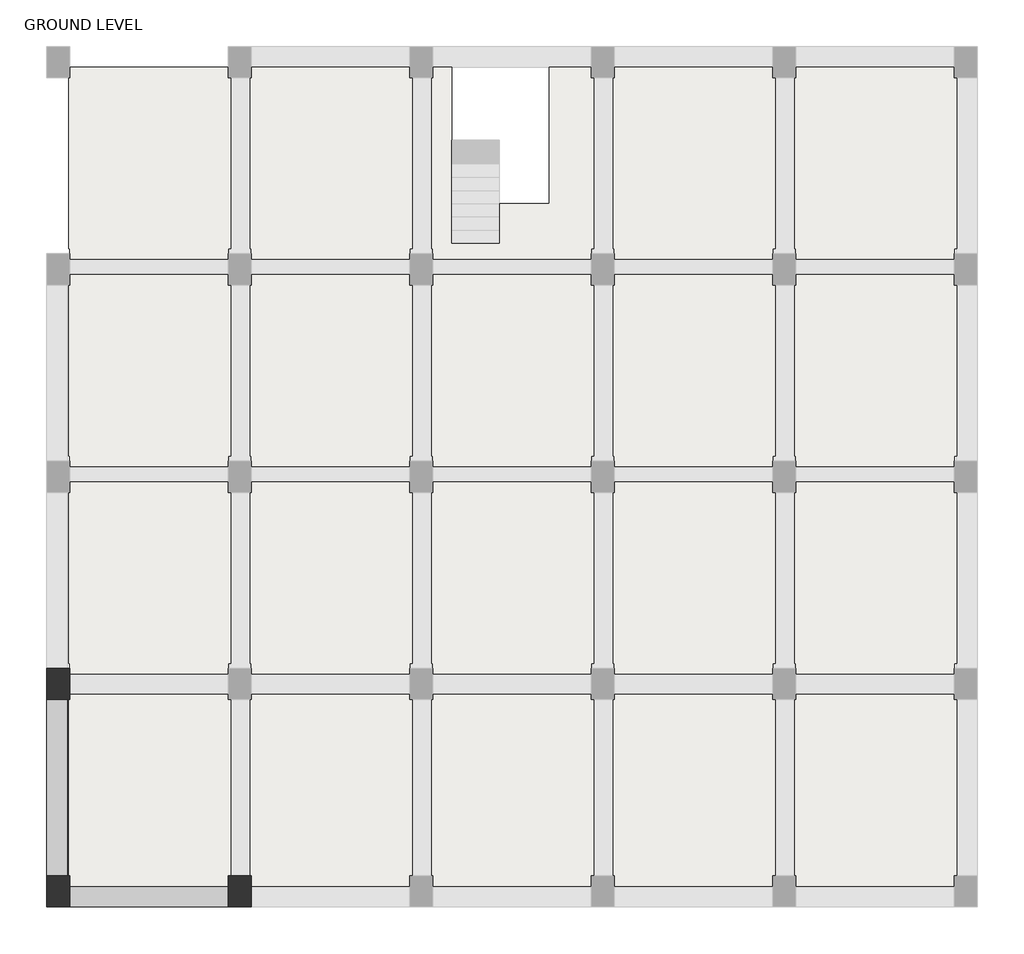
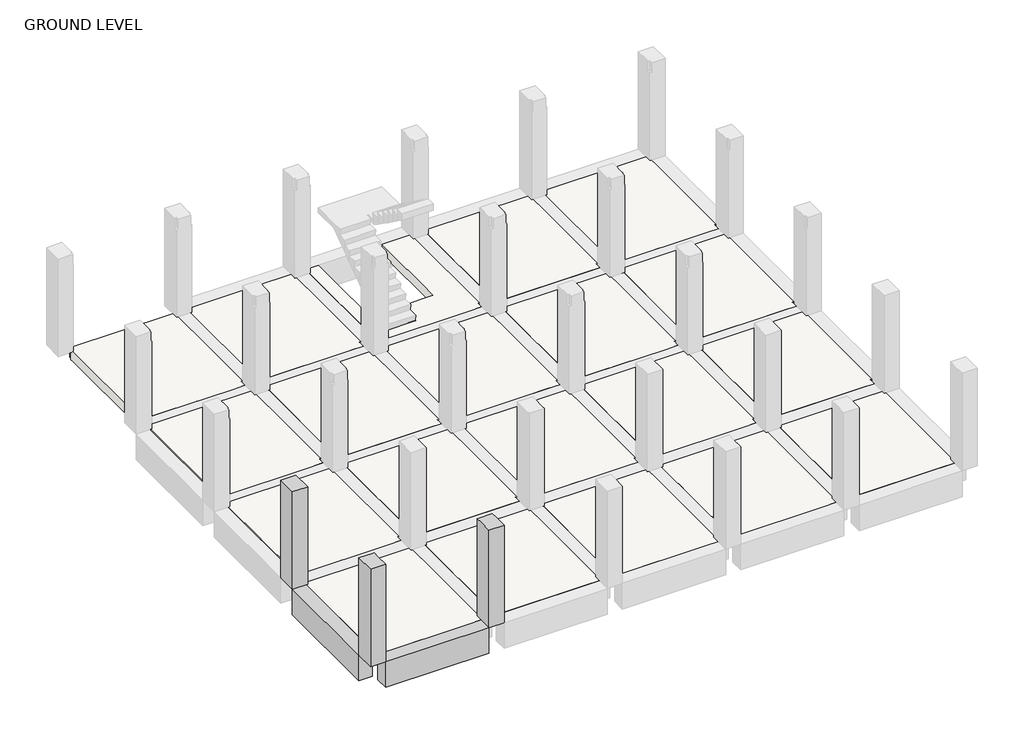
# One storey, part 1 of 3: 20 slabs, 3 columns, 2 beams.
"""IFC4 building model written with IfcOpenShell, lengths in millimetres."""

from ifc_helpers import new_model, si_unit, frame, origin, place, context, project, spatial, polyline, outline, extrude, faceted_brep, element, save

model = new_model("IFC4")

# Units and contexts
model_context = context("Model", 3, world=origin())
ifc_project = project(units=[si_unit("LENGTHUNIT", "METRE", prefix="MILLI")], contexts=[model_context])

# Site, building, storey
site = spatial("IfcSite", under=ifc_project)
building = spatial("IfcBuilding", under=site)
storey = spatial("IfcBuildingStorey", under=building, Name="GROUND LEVEL", Elevation=0.0)

# Beams
placement = place(None, origin())
element("IfcBeam", 1, ObjectType="M_Concrete-Rectangular Beam : 400 x 800mm", at=placement, inside=storey, context=model_context, shape_type="Brep", body=[
    faceted_brep([(-9144.8884094, 3503.1212443, 0.0), (-9144.8884094, 3103.1212443, 0.0), (-6094.8884094, 3103.1212443, 0.0), (-6094.8884094, 3503.1212443, 0.0), (-9144.8884094, 3503.1212443, -800.0), (-9144.8884094, 3503.1212443, -300.0), (-6094.8884094, 3503.1212443, -300.0), (-6094.8884094, 3503.1212443, -800.0), (-9144.8884094, 3103.1212443, -800.0), (-6094.8884094, 3103.1212443, -800.0)], [[[0, 1, 2, 3]], [[4, 5, 0, 3, 6, 7]], [[8, 4, 7, 9]], [[1, 8, 9, 2]], [[1, 0, 5, 4, 8]], [[3, 2, 9, 7, 6]]]),
])
element("IfcBeam", 2, ObjectType="M_Concrete-Rectangular Beam : 400 x 800mm", at=placement, inside=storey, context=model_context, shape_type="SweptSolid", body=[
    extrude(outline(polyline([(-9594.8884094, 7103.1212443), (-9194.8884094, 7103.1212443), (-9194.8884094, 3703.1212443), (-9594.8884094, 3703.1212443), (-9594.8884094, 7103.1212443)])), frame((0.0, 0.0, -800.0), z_axis=(0.0, 0.0, 1.0), x_axis=(1.0, 0.0, 0.0)), (0.0, 0.0, 1.0), 800.0),
])

# Columns
element("IfcColumn", 3, ObjectType="M_Concrete-Rectangular-Column : 450 x 600mm", at=placement, inside=storey, context=model_context, shape_type="Brep", body=[
    faceted_brep([(-9144.8884094, 7703.1212443, 0.0), (-9144.8884094, 7103.1212443, 0.0), (-9594.8884094, 7103.1212443, 0.0), (-9594.8884094, 7703.1212443, 0.0), (-9144.8884094, 7703.1212443, 2748.0), (-9144.8884094, 7703.1212443, 3048.0), (-9144.8884094, 7603.1212443, 3048.0), (-9144.8884094, 7203.1212443, 3048.0), (-9144.8884094, 7103.1212443, 3048.0), (-9144.8884094, 7103.1212443, 2748.0), (-9169.8884094, 7103.1212443, 3048.0), (-9594.8884094, 7103.1212443, 3048.0), (-9594.8884094, 7703.1212443, 3048.0)], [[[0, 1, 2, 3]], [[1, 0, 4, 5, 6, 7, 8, 9]], [[2, 1, 9, 8, 10, 11]], [[3, 2, 11, 12]], [[0, 3, 12, 5, 4]], [[12, 11, 10, 8, 7, 6, 5]]]),
])
element("IfcColumn", 4, ObjectType="M_Concrete-Rectangular-Column : 450 x 600mm", at=placement, inside=storey, context=model_context, shape_type="Brep", body=[
    faceted_brep([(-9144.8884094, 3703.1212443, 0.0), (-9144.8884094, 3103.1212443, 0.0), (-9594.8884094, 3103.1212443, 0.0), (-9594.8884094, 3703.1212443, 0.0), (-9144.8884094, 3703.1212443, 2748.0), (-9144.8884094, 3703.1212443, 3048.0), (-9144.8884094, 3503.1212443, 3048.0), (-9144.8884094, 3103.1212443, 3048.0), (-9594.8884094, 3103.1212443, 3048.0), (-9594.8884094, 3703.1212443, 3048.0), (-9169.8884094, 3703.1212443, 3048.0)], [[[0, 1, 2, 3]], [[1, 0, 4, 5, 6, 7]], [[2, 1, 7, 8]], [[3, 2, 8, 9]], [[0, 3, 9, 10, 5, 4]], [[8, 7, 6, 5, 10, 9]]]),
])
element("IfcColumn", 5, ObjectType="M_Concrete-Rectangular-Column : 450 x 600mm", at=placement, inside=storey, context=model_context, shape_type="Brep", body=[
    faceted_brep([(-5644.8884094, 3703.1212443, 0.0), (-5644.8884094, 3103.1212443, 0.0), (-6094.8884094, 3103.1212443, 0.0), (-6094.8884094, 3703.1212443, 0.0), (-5644.8884094, 3703.1212443, 2748.0), (-5644.8884094, 3703.1212443, 3048.0), (-5644.8884094, 3503.1212443, 3048.0), (-5644.8884094, 3103.1212443, 3048.0), (-6094.8884094, 3103.1212443, 3048.0), (-6094.8884094, 3503.1212443, 3048.0), (-6094.8884094, 3703.1212443, 3048.0), (-6094.8884094, 3703.1212443, 2748.0), (-6044.8884094, 3703.1212443, 3048.0), (-5669.8884094, 3703.1212443, 3048.0)], [[[0, 1, 2, 3]], [[1, 0, 4, 5, 6, 7]], [[2, 1, 7, 8]], [[3, 2, 8, 9, 10, 11]], [[0, 3, 11, 10, 12, 13, 5, 4]], [[8, 7, 6, 5, 13, 12, 10, 9]]]),
])

# Slabs
element("IfcSlab", 6, ObjectType="Generic 300mm", at=placement, inside=storey, context=model_context, shape_type="SweptSolid", body=[
    extrude(outline(polyline([(7955.1115906, 7103.1212443), (7955.1115906, 3703.1212443), (7905.1115906, 3703.1212443), (7905.1115906, 3503.1212443), (7530.1115906, 3503.1212443), (4855.1115906, 3503.1212443), (4855.1115906, 3703.1212443), (4830.1115906, 3703.1212443), (4830.1115906, 7103.1212443), (4855.1115906, 7103.1212443), (4855.1115906, 7203.1212443), (7905.1115906, 7203.1212443), (7905.1115906, 7103.1212443), (7955.1115906, 7103.1212443)])), frame((0.0, 0.0, -300.0), z_axis=(0.0, 0.0, 1.0), x_axis=(1.0, 0.0, 0.0)), (0.0, 0.0, 1.0), 300.0),
])
element("IfcSlab", 7, ObjectType="Generic 300mm", at=placement, inside=storey, context=model_context, shape_type="Brep", body=[
    faceted_brep([(7955.1115906, 11203.1212443, -300.0), (7955.1115906, 11103.1212443, -300.0), (7955.1115906, 7803.1212443, -300.0), (7905.1115906, 7803.1212443, -300.0), (7905.1115906, 7603.1212443, -300.0), (7530.1115906, 7603.1212443, -300.0), (4855.1115906, 7603.1212443, -300.0), (4855.1115906, 7803.1212443, -300.0), (4830.1115906, 7803.1212443, -300.0), (4830.1115906, 11103.1212443, -300.0), (4830.1115906, 11203.1212443, -300.0), (4855.1115906, 11203.1212443, -300.0), (4855.1115906, 11303.1212443, -300.0), (7905.1115906, 11303.1212443, -300.0), (7905.1115906, 11203.1212443, -300.0), (7955.1115906, 11203.1212443, 0.0), (7905.1115906, 11203.1212443, 0.0), (7905.1115906, 11303.1212443, 0.0), (4855.1115906, 11303.1212443, 0.0), (4855.1115906, 11203.1212443, 0.0), (4830.1115906, 11203.1212443, 0.0), (4830.1115906, 11103.1212443, 0.0), (4830.1115906, 7803.1212443, 0.0), (4855.1115906, 7803.1212443, 0.0), (4855.1115906, 7703.1212443, 0.0), (4855.1115906, 7603.1212443, 0.0), (7530.1115906, 7603.1212443, 0.0), (7905.1115906, 7603.1212443, 0.0), (7905.1115906, 7703.1212443, 0.0), (7905.1115906, 7803.1212443, 0.0), (7955.1115906, 7803.1212443, 0.0), (7955.1115906, 11103.1212443, 0.0)], [[[0, 1, 2, 3, 4, 5, 6, 7, 8, 9, 10, 11, 12, 13, 14]], [[15, 16, 17, 18, 19, 20, 21, 22, 23, 24, 25, 26, 27, 28, 29, 30, 31]], [[2, 1, 0, 15, 31, 30]], [[3, 2, 30, 29]], [[4, 3, 29, 28, 27]], [[5, 4, 27, 26]], [[6, 5, 26, 25]], [[7, 6, 25, 24, 23]], [[8, 7, 23, 22]], [[10, 9, 8, 22, 21, 20]], [[11, 10, 20, 19]], [[12, 11, 19, 18]], [[13, 12, 18, 17]], [[14, 13, 17, 16]], [[0, 14, 16, 15]]]),
])
element("IfcSlab", 8, ObjectType="Generic 300mm", at=placement, inside=storey, context=model_context, shape_type="Brep", body=[
    faceted_brep([(4455.1115906, 11203.1212443, -300.0), (4455.1115906, 11103.1212443, -300.0), (4455.1115906, 7803.1212443, -300.0), (4430.1115906, 7803.1212443, -300.0), (4405.1115906, 7803.1212443, -300.0), (4405.1115906, 7603.1212443, -300.0), (4030.1115906, 7603.1212443, -300.0), (1355.1115906, 7603.1212443, -300.0), (1355.1115906, 7803.1212443, -300.0), (1330.1115906, 7803.1212443, -300.0), (1330.1115906, 11103.1212443, -300.0), (1330.1115906, 11203.1212443, -300.0), (1355.1115906, 11203.1212443, -300.0), (1355.1115906, 11303.1212443, -300.0), (4405.1115906, 11303.1212443, -300.0), (4405.1115906, 11203.1212443, -300.0), (4455.1115906, 11203.1212443, 0.0), (4405.1115906, 11203.1212443, 0.0), (4405.1115906, 11303.1212443, 0.0), (1355.1115906, 11303.1212443, 0.0), (1355.1115906, 11203.1212443, 0.0), (1330.1115906, 11203.1212443, 0.0), (1330.1115906, 11103.1212443, 0.0), (1330.1115906, 7803.1212443, 0.0), (1355.1115906, 7803.1212443, 0.0), (1355.1115906, 7703.1212443, 0.0), (1355.1115906, 7603.1212443, 0.0), (4030.1115906, 7603.1212443, 0.0), (4405.1115906, 7603.1212443, 0.0), (4405.1115906, 7703.1212443, 0.0), (4405.1115906, 7803.1212443, 0.0), (4430.1115906, 7803.1212443, 0.0), (4455.1115906, 7803.1212443, 0.0), (4455.1115906, 11103.1212443, 0.0)], [[[0, 1, 2, 3, 4, 5, 6, 7, 8, 9, 10, 11, 12, 13, 14, 15]], [[16, 17, 18, 19, 20, 21, 22, 23, 24, 25, 26, 27, 28, 29, 30, 31, 32, 33]], [[2, 1, 0, 16, 33, 32]], [[4, 3, 2, 32, 31, 30]], [[5, 4, 30, 29, 28]], [[6, 5, 28, 27]], [[7, 6, 27, 26]], [[8, 7, 26, 25, 24]], [[9, 8, 24, 23]], [[11, 10, 9, 23, 22, 21]], [[12, 11, 21, 20]], [[13, 12, 20, 19]], [[14, 13, 19, 18]], [[15, 14, 18, 17]], [[0, 15, 17, 16]]]),
])
element("IfcSlab", 9, ObjectType="Generic 300mm", at=placement, inside=storey, context=model_context, shape_type="Brep", body=[
    faceted_brep([(955.1115906, 11203.1212443, -300.0), (955.1115906, 11103.1212443, -300.0), (955.1115906, 7803.1212443, -300.0), (930.1115906, 7803.1212443, -300.0), (905.1115906, 7803.1212443, -300.0), (905.1115906, 7603.1212443, -300.0), (530.1115906, 7603.1212443, -300.0), (-2144.8884094, 7603.1212443, -300.0), (-2144.8884094, 7803.1212443, -300.0), (-2169.8884094, 7803.1212443, -300.0), (-2169.8884094, 11103.1212443, -300.0), (-2169.8884094, 11203.1212443, -300.0), (-2144.8884094, 11203.1212443, -300.0), (-2144.8884094, 11303.1212443, -300.0), (905.1115906, 11303.1212443, -300.0), (905.1115906, 11203.1212443, -300.0), (955.1115906, 11203.1212443, 0.0), (905.1115906, 11203.1212443, 0.0), (905.1115906, 11303.1212443, 0.0), (-2144.8884094, 11303.1212443, 0.0), (-2144.8884094, 11203.1212443, 0.0), (-2169.8884094, 11203.1212443, 0.0), (-2169.8884094, 11103.1212443, 0.0), (-2169.8884094, 7803.1212443, 0.0), (-2144.8884094, 7803.1212443, 0.0), (-2144.8884094, 7703.1212443, 0.0), (-2144.8884094, 7603.1212443, 0.0), (530.1115906, 7603.1212443, 0.0), (905.1115906, 7603.1212443, 0.0), (905.1115906, 7703.1212443, 0.0), (905.1115906, 7803.1212443, 0.0), (930.1115906, 7803.1212443, 0.0), (955.1115906, 7803.1212443, 0.0), (955.1115906, 11103.1212443, 0.0)], [[[0, 1, 2, 3, 4, 5, 6, 7, 8, 9, 10, 11, 12, 13, 14, 15]], [[16, 17, 18, 19, 20, 21, 22, 23, 24, 25, 26, 27, 28, 29, 30, 31, 32, 33]], [[2, 1, 0, 16, 33, 32]], [[4, 3, 2, 32, 31, 30]], [[5, 4, 30, 29, 28]], [[6, 5, 28, 27]], [[7, 6, 27, 26]], [[8, 7, 26, 25, 24]], [[9, 8, 24, 23]], [[11, 10, 9, 23, 22, 21]], [[12, 11, 21, 20]], [[13, 12, 20, 19]], [[14, 13, 19, 18]], [[15, 14, 18, 17]], [[0, 15, 17, 16]]]),
])
element("IfcSlab", 10, ObjectType="Generic 300mm", at=placement, inside=storey, context=model_context, shape_type="Brep", body=[
    faceted_brep([(-2544.8884094, 11203.1212443, -300.0), (-2544.8884094, 11103.1212443, -300.0), (-2544.8884094, 7803.1212443, -300.0), (-2569.8884094, 7803.1212443, -300.0), (-2594.8884094, 7803.1212443, -300.0), (-2594.8884094, 7603.1212443, -300.0), (-2969.8884094, 7603.1212443, -300.0), (-5644.8884094, 7603.1212443, -300.0), (-5644.8884094, 7803.1212443, -300.0), (-5669.8884094, 7803.1212443, -300.0), (-5669.8884094, 11103.1212443, -300.0), (-5669.8884094, 11203.1212443, -300.0), (-5644.8884094, 11203.1212443, -300.0), (-5644.8884094, 11303.1212443, -300.0), (-2594.8884094, 11303.1212443, -300.0), (-2594.8884094, 11203.1212443, -300.0), (-2544.8884094, 11203.1212443, 0.0), (-2594.8884094, 11203.1212443, 0.0), (-2594.8884094, 11303.1212443, 0.0), (-5644.8884094, 11303.1212443, 0.0), (-5644.8884094, 11203.1212443, 0.0), (-5669.8884094, 11203.1212443, 0.0), (-5669.8884094, 11103.1212443, 0.0), (-5669.8884094, 7803.1212443, 0.0), (-5644.8884094, 7803.1212443, 0.0), (-5644.8884094, 7703.1212443, 0.0), (-5644.8884094, 7603.1212443, 0.0), (-2969.8884094, 7603.1212443, 0.0), (-2594.8884094, 7603.1212443, 0.0), (-2594.8884094, 7703.1212443, 0.0), (-2594.8884094, 7803.1212443, 0.0), (-2569.8884094, 7803.1212443, 0.0), (-2544.8884094, 7803.1212443, 0.0), (-2544.8884094, 11103.1212443, 0.0)], [[[0, 1, 2, 3, 4, 5, 6, 7, 8, 9, 10, 11, 12, 13, 14, 15]], [[16, 17, 18, 19, 20, 21, 22, 23, 24, 25, 26, 27, 28, 29, 30, 31, 32, 33]], [[2, 1, 0, 16, 33, 32]], [[4, 3, 2, 32, 31, 30]], [[5, 4, 30, 29, 28]], [[6, 5, 28, 27]], [[7, 6, 27, 26]], [[8, 7, 26, 25, 24]], [[9, 8, 24, 23]], [[11, 10, 9, 23, 22, 21]], [[12, 11, 21, 20]], [[13, 12, 20, 19]], [[14, 13, 19, 18]], [[15, 14, 18, 17]], [[0, 15, 17, 16]]]),
])
element("IfcSlab", 11, ObjectType="Generic 300mm", at=placement, inside=storey, context=model_context, shape_type="Brep", body=[
    faceted_brep([(-6044.8884094, 11203.1212443, -300.0), (-6044.8884094, 11103.1212443, -300.0), (-6044.8884094, 7803.1212443, -300.0), (-6069.8884094, 7803.1212443, -300.0), (-6094.8884094, 7803.1212443, -300.0), (-6094.8884094, 7603.1212443, -300.0), (-6469.8884094, 7603.1212443, -300.0), (-9144.8884094, 7603.1212443, -300.0), (-9144.8884094, 7803.1212443, -300.0), (-9169.8884094, 7803.1212443, -300.0), (-9169.8884094, 11103.1212443, -300.0), (-9169.8884094, 11203.1212443, -300.0), (-9144.8884094, 11203.1212443, -300.0), (-9144.8884094, 11303.1212443, -300.0), (-6094.8884094, 11303.1212443, -300.0), (-6094.8884094, 11203.1212443, -300.0), (-6044.8884094, 11203.1212443, 0.0), (-6094.8884094, 11203.1212443, 0.0), (-6094.8884094, 11303.1212443, 0.0), (-9144.8884094, 11303.1212443, 0.0), (-9144.8884094, 11203.1212443, 0.0), (-9169.8884094, 11203.1212443, 0.0), (-9169.8884094, 11103.1212443, 0.0), (-9169.8884094, 7803.1212443, 0.0), (-9144.8884094, 7803.1212443, 0.0), (-9144.8884094, 7703.1212443, 0.0), (-9144.8884094, 7603.1212443, 0.0), (-6469.8884094, 7603.1212443, 0.0), (-6094.8884094, 7603.1212443, 0.0), (-6094.8884094, 7703.1212443, 0.0), (-6094.8884094, 7803.1212443, 0.0), (-6069.8884094, 7803.1212443, 0.0), (-6044.8884094, 7803.1212443, 0.0), (-6044.8884094, 11103.1212443, 0.0)], [[[0, 1, 2, 3, 4, 5, 6, 7, 8, 9, 10, 11, 12, 13, 14, 15]], [[16, 17, 18, 19, 20, 21, 22, 23, 24, 25, 26, 27, 28, 29, 30, 31, 32, 33]], [[2, 1, 0, 16, 33, 32]], [[4, 3, 2, 32, 31, 30]], [[5, 4, 30, 29, 28]], [[6, 5, 28, 27]], [[7, 6, 27, 26]], [[8, 7, 26, 25, 24]], [[9, 8, 24, 23]], [[11, 10, 9, 23, 22, 21]], [[12, 11, 21, 20]], [[13, 12, 20, 19]], [[14, 13, 19, 18]], [[15, 14, 18, 17]], [[0, 15, 17, 16]]]),
])
element("IfcSlab", 12, ObjectType="Generic 300mm", at=placement, inside=storey, context=model_context, shape_type="Brep", body=[
    faceted_brep([(-6044.8884094, 7103.1212443, -300.0), (-6044.8884094, 3703.1212443, -300.0), (-6069.8884094, 3703.1212443, -300.0), (-6094.8884094, 3703.1212443, -300.0), (-6094.8884094, 3503.1212443, -300.0), (-6469.8884094, 3503.1212443, -300.0), (-9144.8884094, 3503.1212443, -300.0), (-9144.8884094, 3703.1212443, -300.0), (-9169.8884094, 3703.1212443, -300.0), (-9169.8884094, 7103.1212443, -300.0), (-9144.8884094, 7103.1212443, -300.0), (-9144.8884094, 7203.1212443, -300.0), (-6094.8884094, 7203.1212443, -300.0), (-6094.8884094, 7103.1212443, -300.0), (-6069.8884094, 7103.1212443, -300.0), (-6044.8884094, 7103.1212443, 0.0), (-6094.8884094, 7103.1212443, 0.0), (-6094.8884094, 7203.1212443, 0.0), (-9144.8884094, 7203.1212443, 0.0), (-9144.8884094, 7103.1212443, 0.0), (-9169.8884094, 7103.1212443, 0.0), (-9169.8884094, 3703.1212443, 0.0), (-9144.8884094, 3703.1212443, 0.0), (-9144.8884094, 3503.1212443, 0.0), (-6469.8884094, 3503.1212443, 0.0), (-6094.8884094, 3503.1212443, 0.0), (-6094.8884094, 3703.1212443, 0.0), (-6044.8884094, 3703.1212443, 0.0)], [[[0, 1, 2, 3, 4, 5, 6, 7, 8, 9, 10, 11, 12, 13, 14]], [[15, 16, 17, 18, 19, 20, 21, 22, 23, 24, 25, 26, 27]], [[1, 0, 15, 27]], [[3, 2, 1, 27, 26]], [[4, 3, 26, 25]], [[5, 4, 25, 24]], [[6, 5, 24, 23]], [[7, 6, 23, 22]], [[8, 7, 22, 21]], [[9, 8, 21, 20]], [[10, 9, 20, 19]], [[11, 10, 19, 18]], [[12, 11, 18, 17]], [[13, 12, 17, 16]], [[0, 14, 13, 16, 15]]]),
])
element("IfcSlab", 13, ObjectType="Generic 300mm", at=placement, inside=storey, context=model_context, shape_type="Brep", body=[
    faceted_brep([(-2544.8884094, 7103.1212443, -300.0), (-2544.8884094, 3703.1212443, -300.0), (-2569.8884094, 3703.1212443, -300.0), (-2594.8884094, 3703.1212443, -300.0), (-2594.8884094, 3503.1212443, -300.0), (-2969.8884094, 3503.1212443, -300.0), (-5644.8884094, 3503.1212443, -300.0), (-5644.8884094, 3703.1212443, -300.0), (-5669.8884094, 3703.1212443, -300.0), (-5669.8884094, 7103.1212443, -300.0), (-5644.8884094, 7103.1212443, -300.0), (-5644.8884094, 7203.1212443, -300.0), (-2594.8884094, 7203.1212443, -300.0), (-2594.8884094, 7103.1212443, -300.0), (-2569.8884094, 7103.1212443, -300.0), (-2544.8884094, 7103.1212443, 0.0), (-2594.8884094, 7103.1212443, 0.0), (-2594.8884094, 7203.1212443, 0.0), (-5644.8884094, 7203.1212443, 0.0), (-5644.8884094, 7103.1212443, 0.0), (-5669.8884094, 7103.1212443, 0.0), (-5669.8884094, 3703.1212443, 0.0), (-5644.8884094, 3703.1212443, 0.0), (-5644.8884094, 3503.1212443, 0.0), (-2969.8884094, 3503.1212443, 0.0), (-2594.8884094, 3503.1212443, 0.0), (-2594.8884094, 3703.1212443, 0.0), (-2544.8884094, 3703.1212443, 0.0)], [[[0, 1, 2, 3, 4, 5, 6, 7, 8, 9, 10, 11, 12, 13, 14]], [[15, 16, 17, 18, 19, 20, 21, 22, 23, 24, 25, 26, 27]], [[1, 0, 15, 27]], [[3, 2, 1, 27, 26]], [[4, 3, 26, 25]], [[5, 4, 25, 24]], [[6, 5, 24, 23]], [[7, 6, 23, 22]], [[8, 7, 22, 21]], [[9, 8, 21, 20]], [[10, 9, 20, 19]], [[11, 10, 19, 18]], [[12, 11, 18, 17]], [[13, 12, 17, 16]], [[0, 14, 13, 16, 15]]]),
])
element("IfcSlab", 14, ObjectType="Generic 300mm", at=placement, inside=storey, context=model_context, shape_type="Brep", body=[
    faceted_brep([(955.1115906, 7103.1212443, -300.0), (955.1115906, 3703.1212443, -300.0), (930.1115906, 3703.1212443, -300.0), (905.1115906, 3703.1212443, -300.0), (905.1115906, 3503.1212443, -300.0), (530.1115906, 3503.1212443, -300.0), (-2144.8884094, 3503.1212443, -300.0), (-2144.8884094, 3703.1212443, -300.0), (-2169.8884094, 3703.1212443, -300.0), (-2169.8884094, 7103.1212443, -300.0), (-2144.8884094, 7103.1212443, -300.0), (-2144.8884094, 7203.1212443, -300.0), (905.1115906, 7203.1212443, -300.0), (905.1115906, 7103.1212443, -300.0), (930.1115906, 7103.1212443, -300.0), (955.1115906, 7103.1212443, 0.0), (905.1115906, 7103.1212443, 0.0), (905.1115906, 7203.1212443, 0.0), (-2144.8884094, 7203.1212443, 0.0), (-2144.8884094, 7103.1212443, 0.0), (-2169.8884094, 7103.1212443, 0.0), (-2169.8884094, 3703.1212443, 0.0), (-2144.8884094, 3703.1212443, 0.0), (-2144.8884094, 3503.1212443, 0.0), (530.1115906, 3503.1212443, 0.0), (905.1115906, 3503.1212443, 0.0), (905.1115906, 3703.1212443, 0.0), (955.1115906, 3703.1212443, 0.0)], [[[0, 1, 2, 3, 4, 5, 6, 7, 8, 9, 10, 11, 12, 13, 14]], [[15, 16, 17, 18, 19, 20, 21, 22, 23, 24, 25, 26, 27]], [[1, 0, 15, 27]], [[3, 2, 1, 27, 26]], [[4, 3, 26, 25]], [[5, 4, 25, 24]], [[6, 5, 24, 23]], [[7, 6, 23, 22]], [[8, 7, 22, 21]], [[9, 8, 21, 20]], [[10, 9, 20, 19]], [[11, 10, 19, 18]], [[12, 11, 18, 17]], [[13, 12, 17, 16]], [[0, 14, 13, 16, 15]]]),
])
element("IfcSlab", 15, ObjectType="Generic 300mm", at=placement, inside=storey, context=model_context, shape_type="Brep", body=[
    faceted_brep([(4455.1115906, 7103.1212443, -300.0), (4455.1115906, 3703.1212443, -300.0), (4430.1115906, 3703.1212443, -300.0), (4405.1115906, 3703.1212443, -300.0), (4405.1115906, 3503.1212443, -300.0), (4030.1115906, 3503.1212443, -300.0), (1355.1115906, 3503.1212443, -300.0), (1355.1115906, 3703.1212443, -300.0), (1330.1115906, 3703.1212443, -300.0), (1330.1115906, 7103.1212443, -300.0), (1355.1115906, 7103.1212443, -300.0), (1355.1115906, 7203.1212443, -300.0), (4405.1115906, 7203.1212443, -300.0), (4405.1115906, 7103.1212443, -300.0), (4430.1115906, 7103.1212443, -300.0), (4455.1115906, 7103.1212443, 0.0), (4405.1115906, 7103.1212443, 0.0), (4405.1115906, 7203.1212443, 0.0), (1355.1115906, 7203.1212443, 0.0), (1355.1115906, 7103.1212443, 0.0), (1330.1115906, 7103.1212443, 0.0), (1330.1115906, 3703.1212443, 0.0), (1355.1115906, 3703.1212443, 0.0), (1355.1115906, 3503.1212443, 0.0), (4030.1115906, 3503.1212443, 0.0), (4405.1115906, 3503.1212443, 0.0), (4405.1115906, 3703.1212443, 0.0), (4455.1115906, 3703.1212443, 0.0)], [[[0, 1, 2, 3, 4, 5, 6, 7, 8, 9, 10, 11, 12, 13, 14]], [[15, 16, 17, 18, 19, 20, 21, 22, 23, 24, 25, 26, 27]], [[1, 0, 15, 27]], [[3, 2, 1, 27, 26]], [[4, 3, 26, 25]], [[5, 4, 25, 24]], [[6, 5, 24, 23]], [[7, 6, 23, 22]], [[8, 7, 22, 21]], [[9, 8, 21, 20]], [[10, 9, 20, 19]], [[11, 10, 19, 18]], [[12, 11, 18, 17]], [[13, 12, 17, 16]], [[0, 14, 13, 16, 15]]]),
])
element("IfcSlab", 16, ObjectType="Generic 300mm", at=placement, inside=storey, context=model_context, shape_type="Brep", body=[
    faceted_brep([(7955.1115906, 15203.1212443, -300.0), (7955.1115906, 15103.1212443, -300.0), (7955.1115906, 11803.1212443, -300.0), (7905.1115906, 11803.1212443, -300.0), (7905.1115906, 11603.1212443, -300.0), (7530.1115906, 11603.1212443, -300.0), (4855.1115906, 11603.1212443, -300.0), (4855.1115906, 11803.1212443, -300.0), (4830.1115906, 11803.1212443, -300.0), (4830.1115906, 15103.1212443, -300.0), (4830.1115906, 15203.1212443, -300.0), (4855.1115906, 15203.1212443, -300.0), (4855.1115906, 15303.1212443, -300.0), (7905.1115906, 15303.1212443, -300.0), (7905.1115906, 15203.1212443, -300.0), (7955.1115906, 15203.1212443, 0.0), (7905.1115906, 15203.1212443, 0.0), (7905.1115906, 15303.1212443, 0.0), (4855.1115906, 15303.1212443, 0.0), (4855.1115906, 15203.1212443, 0.0), (4830.1115906, 15203.1212443, 0.0), (4830.1115906, 15103.1212443, 0.0), (4830.1115906, 11803.1212443, 0.0), (4855.1115906, 11803.1212443, 0.0), (4855.1115906, 11703.1212443, 0.0), (4855.1115906, 11603.1212443, 0.0), (7530.1115906, 11603.1212443, 0.0), (7905.1115906, 11603.1212443, 0.0), (7905.1115906, 11703.1212443, 0.0), (7905.1115906, 11803.1212443, 0.0), (7955.1115906, 11803.1212443, 0.0), (7955.1115906, 15103.1212443, 0.0)], [[[0, 1, 2, 3, 4, 5, 6, 7, 8, 9, 10, 11, 12, 13, 14]], [[15, 16, 17, 18, 19, 20, 21, 22, 23, 24, 25, 26, 27, 28, 29, 30, 31]], [[2, 1, 0, 15, 31, 30]], [[3, 2, 30, 29]], [[4, 3, 29, 28, 27]], [[5, 4, 27, 26]], [[6, 5, 26, 25]], [[7, 6, 25, 24, 23]], [[8, 7, 23, 22]], [[10, 9, 8, 22, 21, 20]], [[11, 10, 20, 19]], [[12, 11, 19, 18]], [[13, 12, 18, 17]], [[14, 13, 17, 16]], [[0, 14, 16, 15]]]),
])
element("IfcSlab", 17, ObjectType="Generic 300mm", at=placement, inside=storey, context=model_context, shape_type="Brep", body=[
    faceted_brep([(7955.1115906, 19203.1212443, -300.0), (7955.1115906, 19103.1212443, -300.0), (7955.1115906, 15803.1212443, -300.0), (7905.1115906, 15803.1212443, -300.0), (7905.1115906, 15603.1212443, -300.0), (7530.1115906, 15603.1212443, -300.0), (4855.1115906, 15603.1212443, -300.0), (4855.1115906, 15803.1212443, -300.0), (4830.1115906, 15803.1212443, -300.0), (4830.1115906, 19103.1212443, -300.0), (4830.1115906, 19203.1212443, -300.0), (4855.1115906, 19203.1212443, -300.0), (4855.1115906, 19303.1212443, -300.0), (7905.1115906, 19303.1212443, -300.0), (7905.1115906, 19203.1212443, -300.0), (7955.1115906, 19203.1212443, 0.0), (7905.1115906, 19203.1212443, 0.0), (7905.1115906, 19303.1212443, 0.0), (4855.1115906, 19303.1212443, 0.0), (4855.1115906, 19203.1212443, 0.0), (4830.1115906, 19203.1212443, 0.0), (4830.1115906, 19103.1212443, 0.0), (4830.1115906, 15803.1212443, 0.0), (4855.1115906, 15803.1212443, 0.0), (4855.1115906, 15703.1212443, 0.0), (4855.1115906, 15603.1212443, 0.0), (7530.1115906, 15603.1212443, 0.0), (7905.1115906, 15603.1212443, 0.0), (7905.1115906, 15703.1212443, 0.0), (7905.1115906, 15803.1212443, 0.0), (7955.1115906, 15803.1212443, 0.0), (7955.1115906, 19103.1212443, 0.0)], [[[0, 1, 2, 3, 4, 5, 6, 7, 8, 9, 10, 11, 12, 13, 14]], [[15, 16, 17, 18, 19, 20, 21, 22, 23, 24, 25, 26, 27, 28, 29, 30, 31]], [[2, 1, 0, 15, 31, 30]], [[3, 2, 30, 29]], [[4, 3, 29, 28, 27]], [[5, 4, 27, 26]], [[6, 5, 26, 25]], [[7, 6, 25, 24, 23]], [[8, 7, 23, 22]], [[10, 9, 8, 22, 21, 20]], [[11, 10, 20, 19]], [[12, 11, 19, 18]], [[13, 12, 18, 17]], [[14, 13, 17, 16]], [[0, 14, 16, 15]]]),
])
element("IfcSlab", 18, ObjectType="Generic 300mm", at=placement, inside=storey, context=model_context, shape_type="Brep", body=[
    faceted_brep([(4455.1115906, 19203.1212443, -300.0), (4455.1115906, 19103.1212443, -300.0), (4455.1115906, 15803.1212443, -300.0), (4430.1115906, 15803.1212443, -300.0), (4405.1115906, 15803.1212443, -300.0), (4405.1115906, 15603.1212443, -300.0), (4030.1115906, 15603.1212443, -300.0), (1355.1115906, 15603.1212443, -300.0), (1355.1115906, 15803.1212443, -300.0), (1330.1115906, 15803.1212443, -300.0), (1330.1115906, 19103.1212443, -300.0), (1330.1115906, 19203.1212443, -300.0), (1355.1115906, 19203.1212443, -300.0), (1355.1115906, 19303.1212443, -300.0), (4405.1115906, 19303.1212443, -300.0), (4405.1115906, 19203.1212443, -300.0), (4455.1115906, 19203.1212443, 0.0), (4405.1115906, 19203.1212443, 0.0), (4405.1115906, 19303.1212443, 0.0), (1355.1115906, 19303.1212443, 0.0), (1355.1115906, 19203.1212443, 0.0), (1330.1115906, 19203.1212443, 0.0), (1330.1115906, 19103.1212443, 0.0), (1330.1115906, 15803.1212443, 0.0), (1355.1115906, 15803.1212443, 0.0), (1355.1115906, 15703.1212443, 0.0), (1355.1115906, 15603.1212443, 0.0), (4030.1115906, 15603.1212443, 0.0), (4405.1115906, 15603.1212443, 0.0), (4405.1115906, 15703.1212443, 0.0), (4405.1115906, 15803.1212443, 0.0), (4430.1115906, 15803.1212443, 0.0), (4455.1115906, 15803.1212443, 0.0), (4455.1115906, 19103.1212443, 0.0)], [[[0, 1, 2, 3, 4, 5, 6, 7, 8, 9, 10, 11, 12, 13, 14, 15]], [[16, 17, 18, 19, 20, 21, 22, 23, 24, 25, 26, 27, 28, 29, 30, 31, 32, 33]], [[2, 1, 0, 16, 33, 32]], [[4, 3, 2, 32, 31, 30]], [[5, 4, 30, 29, 28]], [[6, 5, 28, 27]], [[7, 6, 27, 26]], [[8, 7, 26, 25, 24]], [[9, 8, 24, 23]], [[11, 10, 9, 23, 22, 21]], [[12, 11, 21, 20]], [[13, 12, 20, 19]], [[14, 13, 19, 18]], [[15, 14, 18, 17]], [[0, 15, 17, 16]]]),
])
element("IfcSlab", 19, ObjectType="Generic 300mm", at=placement, inside=storey, context=model_context, shape_type="Brep", body=[
    faceted_brep([(4455.1115906, 15203.1212443, -300.0), (4455.1115906, 15103.1212443, -300.0), (4455.1115906, 11803.1212443, -300.0), (4430.1115906, 11803.1212443, -300.0), (4405.1115906, 11803.1212443, -300.0), (4405.1115906, 11603.1212443, -300.0), (4030.1115906, 11603.1212443, -300.0), (1355.1115906, 11603.1212443, -300.0), (1355.1115906, 11803.1212443, -300.0), (1330.1115906, 11803.1212443, -300.0), (1330.1115906, 15103.1212443, -300.0), (1330.1115906, 15203.1212443, -300.0), (1355.1115906, 15203.1212443, -300.0), (1355.1115906, 15303.1212443, -300.0), (4405.1115906, 15303.1212443, -300.0), (4405.1115906, 15203.1212443, -300.0), (4455.1115906, 15203.1212443, 0.0), (4405.1115906, 15203.1212443, 0.0), (4405.1115906, 15303.1212443, 0.0), (1355.1115906, 15303.1212443, 0.0), (1355.1115906, 15203.1212443, 0.0), (1330.1115906, 15203.1212443, 0.0), (1330.1115906, 15103.1212443, 0.0), (1330.1115906, 11803.1212443, 0.0), (1355.1115906, 11803.1212443, 0.0), (1355.1115906, 11703.1212443, 0.0), (1355.1115906, 11603.1212443, 0.0), (4030.1115906, 11603.1212443, 0.0), (4405.1115906, 11603.1212443, 0.0), (4405.1115906, 11703.1212443, 0.0), (4405.1115906, 11803.1212443, 0.0), (4430.1115906, 11803.1212443, 0.0), (4455.1115906, 11803.1212443, 0.0), (4455.1115906, 15103.1212443, 0.0)], [[[0, 1, 2, 3, 4, 5, 6, 7, 8, 9, 10, 11, 12, 13, 14, 15]], [[16, 17, 18, 19, 20, 21, 22, 23, 24, 25, 26, 27, 28, 29, 30, 31, 32, 33]], [[2, 1, 0, 16, 33, 32]], [[4, 3, 2, 32, 31, 30]], [[5, 4, 30, 29, 28]], [[6, 5, 28, 27]], [[7, 6, 27, 26]], [[8, 7, 26, 25, 24]], [[9, 8, 24, 23]], [[11, 10, 9, 23, 22, 21]], [[12, 11, 21, 20]], [[13, 12, 20, 19]], [[14, 13, 19, 18]], [[15, 14, 18, 17]], [[0, 15, 17, 16]]]),
])
element("IfcSlab", 20, ObjectType="Generic 300mm", at=placement, inside=storey, context=model_context, shape_type="Brep", body=[
    faceted_brep([(955.1115906, 15203.1212443, -300.0), (955.1115906, 15103.1212443, -300.0), (955.1115906, 11803.1212443, -300.0), (930.1115906, 11803.1212443, -300.0), (905.1115906, 11803.1212443, -300.0), (905.1115906, 11603.1212443, -300.0), (530.1115906, 11603.1212443, -300.0), (-2144.8884094, 11603.1212443, -300.0), (-2144.8884094, 11803.1212443, -300.0), (-2169.8884094, 11803.1212443, -300.0), (-2169.8884094, 15103.1212443, -300.0), (-2169.8884094, 15203.1212443, -300.0), (-2144.8884094, 15203.1212443, -300.0), (-2144.8884094, 15303.1212443, -300.0), (905.1115906, 15303.1212443, -300.0), (905.1115906, 15203.1212443, -300.0), (955.1115906, 15203.1212443, 0.0), (905.1115906, 15203.1212443, 0.0), (905.1115906, 15303.1212443, 0.0), (-2144.8884094, 15303.1212443, 0.0), (-2144.8884094, 15203.1212443, 0.0), (-2169.8884094, 15203.1212443, 0.0), (-2169.8884094, 15103.1212443, 0.0), (-2169.8884094, 11803.1212443, 0.0), (-2144.8884094, 11803.1212443, 0.0), (-2144.8884094, 11703.1212443, 0.0), (-2144.8884094, 11603.1212443, 0.0), (530.1115906, 11603.1212443, 0.0), (905.1115906, 11603.1212443, 0.0), (905.1115906, 11703.1212443, 0.0), (905.1115906, 11803.1212443, 0.0), (930.1115906, 11803.1212443, 0.0), (955.1115906, 11803.1212443, 0.0), (955.1115906, 15103.1212443, 0.0)], [[[0, 1, 2, 3, 4, 5, 6, 7, 8, 9, 10, 11, 12, 13, 14, 15]], [[16, 17, 18, 19, 20, 21, 22, 23, 24, 25, 26, 27, 28, 29, 30, 31, 32, 33]], [[2, 1, 0, 16, 33, 32]], [[4, 3, 2, 32, 31, 30]], [[5, 4, 30, 29, 28]], [[6, 5, 28, 27]], [[7, 6, 27, 26]], [[8, 7, 26, 25, 24]], [[9, 8, 24, 23]], [[11, 10, 9, 23, 22, 21]], [[12, 11, 21, 20]], [[13, 12, 20, 19]], [[14, 13, 19, 18]], [[15, 14, 18, 17]], [[0, 15, 17, 16]]]),
])
element("IfcSlab", 21, ObjectType="Generic 300mm", at=placement, inside=storey, context=model_context, shape_type="Brep", body=[
    faceted_brep([(955.1115906, 19203.1212443, -300.0), (955.1115906, 19103.1212443, -300.0), (955.1115906, 15803.1212443, -300.0), (930.1115906, 15803.1212443, -300.0), (905.1115906, 15803.1212443, -300.0), (905.1115906, 15603.1212443, -300.0), (530.1115906, 15603.1212443, -300.0), (-2144.8884094, 15603.1212443, -300.0), (-2144.8884094, 15803.1212443, -300.0), (-2169.8884094, 15803.1212443, -300.0), (-2169.8884094, 19103.1212443, -300.0), (-2169.8884094, 19203.1212443, -300.0), (-2144.8884094, 19203.1212443, -300.0), (-2144.8884094, 19303.1212443, -300.0), (-1784.8884094, 19303.1212443, -300.0), (-1784.8884094, 15908.7212443, -300.0), (-870.4884094, 15908.7212443, -300.0), (-870.4884094, 16670.7212443, -300.0), (-819.6884094, 16670.7212443, -300.0), (94.7115906, 16670.7212443, -300.0), (94.7115906, 19303.1212443, -300.0), (905.1115906, 19303.1212443, -300.0), (905.1115906, 19203.1212443, -300.0), (955.1115906, 15803.1212443, 0.0), (955.1115906, 19103.1212443, 0.0), (955.1115906, 19203.1212443, 0.0), (905.1115906, 19203.1212443, 0.0), (905.1115906, 19303.1212443, 0.0), (94.7115906, 19303.1212443, 0.0), (94.7115906, 16670.7212443, 0.0), (-819.6884094, 16670.7212443, 0.0), (-870.4884094, 16670.7212443, 0.0), (-870.4884094, 15908.7212443, 0.0), (-1784.8884094, 15908.7212443, 0.0), (-1784.8884094, 19303.1212443, 0.0), (-2144.8884094, 19303.1212443, 0.0), (-2144.8884094, 19203.1212443, 0.0), (-2169.8884094, 19203.1212443, 0.0), (-2169.8884094, 19103.1212443, 0.0), (-2169.8884094, 15803.1212443, 0.0), (-2144.8884094, 15803.1212443, 0.0), (-2144.8884094, 15703.1212443, 0.0), (-2144.8884094, 15603.1212443, 0.0), (530.1115906, 15603.1212443, 0.0), (905.1115906, 15603.1212443, 0.0), (905.1115906, 15703.1212443, 0.0), (905.1115906, 15803.1212443, 0.0), (930.1115906, 15803.1212443, 0.0)], [[[0, 1, 2, 3, 4, 5, 6, 7, 8, 9, 10, 11, 12, 13, 14, 15, 16, 17, 18, 19, 20, 21, 22]], [[23, 24, 25, 26, 27, 28, 29, 30, 31, 32, 33, 34, 35, 36, 37, 38, 39, 40, 41, 42, 43, 44, 45, 46, 47]], [[2, 1, 0, 25, 24, 23]], [[4, 3, 2, 23, 47, 46]], [[5, 4, 46, 45, 44]], [[6, 5, 44, 43]], [[7, 6, 43, 42]], [[8, 7, 42, 41, 40]], [[9, 8, 40, 39]], [[11, 10, 9, 39, 38, 37]], [[12, 11, 37, 36]], [[13, 12, 36, 35]], [[13, 35, 34, 14]], [[27, 21, 20, 28]], [[22, 21, 27, 26]], [[0, 22, 26, 25]], [[19, 29, 28, 20]], [[33, 15, 14, 34]], [[15, 33, 32, 16]], [[16, 32, 31, 17]], [[17, 31, 30, 18]], [[29, 19, 18, 30]]]),
])
element("IfcSlab", 22, ObjectType="Generic 300mm", at=placement, inside=storey, context=model_context, shape_type="Brep", body=[
    faceted_brep([(-2544.8884094, 19203.1212443, -300.0), (-2544.8884094, 19103.1212443, -300.0), (-2544.8884094, 15803.1212443, -300.0), (-2569.8884094, 15803.1212443, -300.0), (-2594.8884094, 15803.1212443, -300.0), (-2594.8884094, 15603.1212443, -300.0), (-2969.8884094, 15603.1212443, -300.0), (-5644.8884094, 15603.1212443, -300.0), (-5644.8884094, 15803.1212443, -300.0), (-5669.8884094, 15803.1212443, -300.0), (-5669.8884094, 19103.1212443, -300.0), (-5669.8884094, 19203.1212443, -300.0), (-5644.8884094, 19203.1212443, -300.0), (-5644.8884094, 19303.1212443, -300.0), (-2594.8884094, 19303.1212443, -300.0), (-2594.8884094, 19203.1212443, -300.0), (-2544.8884094, 19203.1212443, 0.0), (-2594.8884094, 19203.1212443, 0.0), (-2594.8884094, 19303.1212443, 0.0), (-5644.8884094, 19303.1212443, 0.0), (-5644.8884094, 19203.1212443, 0.0), (-5669.8884094, 19203.1212443, 0.0), (-5669.8884094, 19103.1212443, 0.0), (-5669.8884094, 15803.1212443, 0.0), (-5644.8884094, 15803.1212443, 0.0), (-5644.8884094, 15703.1212443, 0.0), (-5644.8884094, 15603.1212443, 0.0), (-2969.8884094, 15603.1212443, 0.0), (-2594.8884094, 15603.1212443, 0.0), (-2594.8884094, 15703.1212443, 0.0), (-2594.8884094, 15803.1212443, 0.0), (-2569.8884094, 15803.1212443, 0.0), (-2544.8884094, 15803.1212443, 0.0), (-2544.8884094, 19103.1212443, 0.0)], [[[0, 1, 2, 3, 4, 5, 6, 7, 8, 9, 10, 11, 12, 13, 14, 15]], [[16, 17, 18, 19, 20, 21, 22, 23, 24, 25, 26, 27, 28, 29, 30, 31, 32, 33]], [[2, 1, 0, 16, 33, 32]], [[4, 3, 2, 32, 31, 30]], [[5, 4, 30, 29, 28]], [[6, 5, 28, 27]], [[7, 6, 27, 26]], [[8, 7, 26, 25, 24]], [[9, 8, 24, 23]], [[11, 10, 9, 23, 22, 21]], [[12, 11, 21, 20]], [[13, 12, 20, 19]], [[14, 13, 19, 18]], [[15, 14, 18, 17]], [[0, 15, 17, 16]]]),
])
element("IfcSlab", 23, ObjectType="Generic 300mm", at=placement, inside=storey, context=model_context, shape_type="Brep", body=[
    faceted_brep([(-6044.8884094, 19203.1212443, -300.0), (-6044.8884094, 19103.1212443, -300.0), (-6044.8884094, 15803.1212443, -300.0), (-6069.8884094, 15803.1212443, -300.0), (-6094.8884094, 15803.1212443, -300.0), (-6094.8884094, 15603.1212443, -300.0), (-6469.8884094, 15603.1212443, -300.0), (-9144.8884094, 15603.1212443, -300.0), (-9144.8884094, 15803.1212443, -300.0), (-9169.8884094, 15803.1212443, -300.0), (-9169.8884094, 19103.1212443, -300.0), (-9169.8884094, 19203.1212443, -300.0), (-9144.8884094, 19203.1212443, -300.0), (-9144.8884094, 19303.1212443, -300.0), (-6094.8884094, 19303.1212443, -300.0), (-6094.8884094, 19203.1212443, -300.0), (-6044.8884094, 19203.1212443, 0.0), (-6094.8884094, 19203.1212443, 0.0), (-6094.8884094, 19303.1212443, 0.0), (-9144.8884094, 19303.1212443, 0.0), (-9144.8884094, 19203.1212443, 0.0), (-9169.8884094, 19203.1212443, 0.0), (-9169.8884094, 19103.1212443, 0.0), (-9169.8884094, 15803.1212443, 0.0), (-9144.8884094, 15803.1212443, 0.0), (-9144.8884094, 15703.1212443, 0.0), (-9144.8884094, 15603.1212443, 0.0), (-6469.8884094, 15603.1212443, 0.0), (-6094.8884094, 15603.1212443, 0.0), (-6094.8884094, 15703.1212443, 0.0), (-6094.8884094, 15803.1212443, 0.0), (-6069.8884094, 15803.1212443, 0.0), (-6044.8884094, 15803.1212443, 0.0), (-6044.8884094, 19103.1212443, 0.0)], [[[0, 1, 2, 3, 4, 5, 6, 7, 8, 9, 10, 11, 12, 13, 14, 15]], [[16, 17, 18, 19, 20, 21, 22, 23, 24, 25, 26, 27, 28, 29, 30, 31, 32, 33]], [[2, 1, 0, 16, 33, 32]], [[4, 3, 2, 32, 31, 30]], [[5, 4, 30, 29, 28]], [[6, 5, 28, 27]], [[7, 6, 27, 26]], [[8, 7, 26, 25, 24]], [[9, 8, 24, 23]], [[11, 10, 9, 23, 22, 21]], [[12, 11, 21, 20]], [[13, 12, 20, 19]], [[14, 13, 19, 18]], [[15, 14, 18, 17]], [[0, 15, 17, 16]]]),
])
element("IfcSlab", 24, ObjectType="Generic 300mm", at=placement, inside=storey, context=model_context, shape_type="Brep", body=[
    faceted_brep([(-6044.8884094, 15203.1212443, -300.0), (-6044.8884094, 15103.1212443, -300.0), (-6044.8884094, 11803.1212443, -300.0), (-6069.8884094, 11803.1212443, -300.0), (-6094.8884094, 11803.1212443, -300.0), (-6094.8884094, 11603.1212443, -300.0), (-6469.8884094, 11603.1212443, -300.0), (-9144.8884094, 11603.1212443, -300.0), (-9144.8884094, 11803.1212443, -300.0), (-9169.8884094, 11803.1212443, -300.0), (-9169.8884094, 15103.1212443, -300.0), (-9169.8884094, 15203.1212443, -300.0), (-9144.8884094, 15203.1212443, -300.0), (-9144.8884094, 15303.1212443, -300.0), (-6094.8884094, 15303.1212443, -300.0), (-6094.8884094, 15203.1212443, -300.0), (-6044.8884094, 15203.1212443, 0.0), (-6094.8884094, 15203.1212443, 0.0), (-6094.8884094, 15303.1212443, 0.0), (-9144.8884094, 15303.1212443, 0.0), (-9144.8884094, 15203.1212443, 0.0), (-9169.8884094, 15203.1212443, 0.0), (-9169.8884094, 15103.1212443, 0.0), (-9169.8884094, 11803.1212443, 0.0), (-9144.8884094, 11803.1212443, 0.0), (-9144.8884094, 11703.1212443, 0.0), (-9144.8884094, 11603.1212443, 0.0), (-6469.8884094, 11603.1212443, 0.0), (-6094.8884094, 11603.1212443, 0.0), (-6094.8884094, 11703.1212443, 0.0), (-6094.8884094, 11803.1212443, 0.0), (-6069.8884094, 11803.1212443, 0.0), (-6044.8884094, 11803.1212443, 0.0), (-6044.8884094, 15103.1212443, 0.0)], [[[0, 1, 2, 3, 4, 5, 6, 7, 8, 9, 10, 11, 12, 13, 14, 15]], [[16, 17, 18, 19, 20, 21, 22, 23, 24, 25, 26, 27, 28, 29, 30, 31, 32, 33]], [[2, 1, 0, 16, 33, 32]], [[4, 3, 2, 32, 31, 30]], [[5, 4, 30, 29, 28]], [[6, 5, 28, 27]], [[7, 6, 27, 26]], [[8, 7, 26, 25, 24]], [[9, 8, 24, 23]], [[11, 10, 9, 23, 22, 21]], [[12, 11, 21, 20]], [[13, 12, 20, 19]], [[14, 13, 19, 18]], [[15, 14, 18, 17]], [[0, 15, 17, 16]]]),
])
element("IfcSlab", 25, ObjectType="Generic 300mm", at=placement, inside=storey, context=model_context, shape_type="Brep", body=[
    faceted_brep([(-2544.8884094, 15203.1212443, -300.0), (-2544.8884094, 15103.1212443, -300.0), (-2544.8884094, 11803.1212443, -300.0), (-2569.8884094, 11803.1212443, -300.0), (-2594.8884094, 11803.1212443, -300.0), (-2594.8884094, 11603.1212443, -300.0), (-2969.8884094, 11603.1212443, -300.0), (-5644.8884094, 11603.1212443, -300.0), (-5644.8884094, 11803.1212443, -300.0), (-5669.8884094, 11803.1212443, -300.0), (-5669.8884094, 15103.1212443, -300.0), (-5669.8884094, 15203.1212443, -300.0), (-5644.8884094, 15203.1212443, -300.0), (-5644.8884094, 15303.1212443, -300.0), (-2594.8884094, 15303.1212443, -300.0), (-2594.8884094, 15203.1212443, -300.0), (-2544.8884094, 15203.1212443, 0.0), (-2594.8884094, 15203.1212443, 0.0), (-2594.8884094, 15303.1212443, 0.0), (-5644.8884094, 15303.1212443, 0.0), (-5644.8884094, 15203.1212443, 0.0), (-5669.8884094, 15203.1212443, 0.0), (-5669.8884094, 15103.1212443, 0.0), (-5669.8884094, 11803.1212443, 0.0), (-5644.8884094, 11803.1212443, 0.0), (-5644.8884094, 11703.1212443, 0.0), (-5644.8884094, 11603.1212443, 0.0), (-2969.8884094, 11603.1212443, 0.0), (-2594.8884094, 11603.1212443, 0.0), (-2594.8884094, 11703.1212443, 0.0), (-2594.8884094, 11803.1212443, 0.0), (-2569.8884094, 11803.1212443, 0.0), (-2544.8884094, 11803.1212443, 0.0), (-2544.8884094, 15103.1212443, 0.0)], [[[0, 1, 2, 3, 4, 5, 6, 7, 8, 9, 10, 11, 12, 13, 14, 15]], [[16, 17, 18, 19, 20, 21, 22, 23, 24, 25, 26, 27, 28, 29, 30, 31, 32, 33]], [[2, 1, 0, 16, 33, 32]], [[4, 3, 2, 32, 31, 30]], [[5, 4, 30, 29, 28]], [[6, 5, 28, 27]], [[7, 6, 27, 26]], [[8, 7, 26, 25, 24]], [[9, 8, 24, 23]], [[11, 10, 9, 23, 22, 21]], [[12, 11, 21, 20]], [[13, 12, 20, 19]], [[14, 13, 19, 18]], [[15, 14, 18, 17]], [[0, 15, 17, 16]]]),
])

save(model, "model.ifc")

# Revit data of these elements
# Type "M_Concrete-Rectangular Beam : 400 x 800mm"
#   Length [instance default] = 5' - 0"
#   b = 1' - 3.74803"
#   h = 2' - 7.49606"
#   Structural Material [instance default] = Concrete, Cast-in-Place gray
#   Assembly Code = ""
# Type "M_Concrete-Rectangular-Column : 450 x 600mm"
#   b = 1' - 5.71654"
#   h = 1' - 11.62205"
#   Structural Material [instance default] = Concrete, Cast-in-Place gray
# Type "Generic 300mm"
#   Function = 0
#   Layers, outside or top first: 0' - 11.81102" no material (function 1)
# Elements 1, 2 (IfcBeam, "M_Concrete-Rectangular Beam : 400 x 800mm")
#   Structural Material = Concrete, Cast-in-Place gray
#   Phase Created = New Construction
#   Materials on its faces: "Concrete, Cast-in-Place gray"
# Elements 3, 4, 5 (IfcColumn, "M_Concrete-Rectangular-Column : 450 x 600mm")
#   Structural Material = Concrete, Cast-in-Place gray
#   Phase Created = New Construction
#   Materials on its faces: "Concrete, Cast-in-Place gray"
# Elements 6, 7, 8, 9, 10, 11, 12, 13, 14, 15, 16, 17, 18, 19, 20, 21, 22, 23, 24, 25 (IfcSlab, "Generic 300mm")
#   built-in parameter 1001955 = 1.5708 (stored number, unit not read)
#   Height Offset From Level = 0' - 0"
#   built-in parameter 1001954 = 1
#   Phase Created = New Construction
#   Materials on its faces: "Default Floor"
# Materials
#   "Concrete, Cast-in-Place gray": class "Concrete", colour RGB 192 192 192, transparency 0, Description = "Cast-in-place concrete", Cost = 0
#   "Default Floor": colour RGB 127 127 127, transparency 0, Cost = 0
